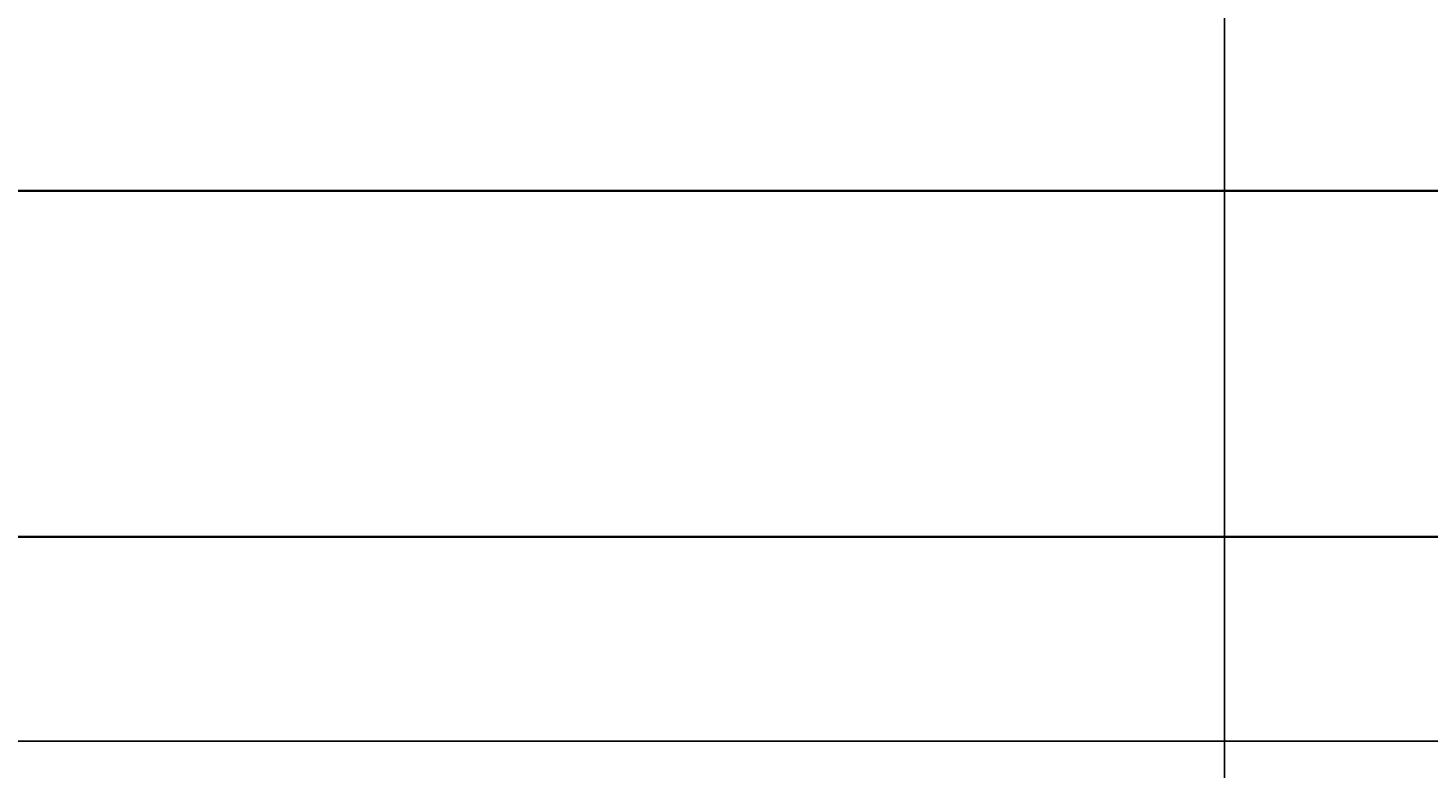
# Model space of a CAD drawing. Units: inches. Extents: x -61 to 1599, y -1316 to 257.
# Tile 49 of 204: x 149 to 185, y -447 to -428. Entities that reach past the tile are written whole.
import ezdxf

# ---------------------------------------------------------------- set-up
doc = ezdxf.new("R2010")
doc.units = ezdxf.units.IN
doc.header["$MEASUREMENT"] = 0
doc.layers.add('A-ANNO-DIMS', color=2, linetype='Continuous', lineweight=18)
doc.layers.add('WALLS', color=4, linetype='Continuous', lineweight=35)
doc.styles.get("Standard").update_dxf_attribs({"font": 'arial.ttf'})
doc.dimstyles.get("Standard").update_dxf_attribs({"dimtxt": 0.18, "dimasz": 0.18, "dimexe": 0.18, "dimexo": 0.0625, "dimgap": 0.09, "dimtad": 0, "dimtih": 1, "dimtoh": 1, "dimdec": 0, "dimzin": 0, "dimdsep": 46, "dimlunit": 3, "dimtxsty": 'Standard', "dimcen": 0.09, "dimadec": 0, "dimazin": 0, "dimtfac": 1, "dimtdec": 0, "dimtofl": 0, "dimtmove": 0, "dimatfit": 3, "dimfxl": 1, "dimtolj": 1, "dimtzin": 0, "dimarcsym": 0})

# ---------------------------------------------------------------- blocks, each defined once
blk = doc.blocks.new('*D687')
at = {"layer": 'A-ANNO-DIMS', "color": 0, "lineweight": -2, "transparency": 16777216}
for p, q in [((289.418, 181.677), (-61.077, 181.677)), ((-60.897, 181.497), (-60.897, -528.952)), ((-60.897, -1239.765), (-60.897, -529.316)), ((319.64, -1239.945), (-61.077, -1239.945))]:
    blk.add_line(p, q, dxfattribs=at)
at = {"layer": 'A-ANNO-DIMS', "color": 0, "transparency": 16777216}
for points in [[(-60.927, 181.497), (-60.867, 181.497), (-60.897, 181.677)], [(-60.927, -1239.765), (-60.867, -1239.765), (-60.897, -1239.945)]]:
    blk.add_solid(points, dxfattribs=at)
at = {"layer": 'DEFPOINTS', "color": 0, "transparency": 16777216}
for p in [(289.481, 181.677), (-60.897, -1239.945), (319.703, -1239.945)]:
    blk.add_point(p, dxfattribs=at)
at = {"layer": 'A-ANNO-DIMS', "color": 0, "transparency": 16777216, "insert": (-60.897, -529.134), "char_height": 0.18, "attachment_point": 5}
blk.add_mtext('\\A1;1421.6', dxfattribs=at)
blk = doc.blocks.new('*D699')
at = {"layer": 'A-ANNO-DIMS', "color": 0, "lineweight": -2, "transparency": 16777216}
for p, q in [((835.64, -167.169), (-61.077, -167.169)), ((-60.897, -167.349), (-60.897, -306.726)), ((-60.897, -446.466), (-60.897, -307.09)), ((841.64, -446.646), (-61.077, -446.646))]:
    blk.add_line(p, q, dxfattribs=at)
at = {"layer": 'A-ANNO-DIMS', "color": 0, "transparency": 16777216}
for points in [[(-60.927, -167.349), (-60.867, -167.349), (-60.897, -167.169)], [(-60.927, -446.466), (-60.867, -446.466), (-60.897, -446.646)]]:
    blk.add_solid(points, dxfattribs=at)
at = {"layer": 'DEFPOINTS', "color": 0, "transparency": 16777216}
for p in [(835.703, -167.169), (-60.897, -446.646), (841.703, -446.646)]:
    blk.add_point(p, dxfattribs=at)
at = {"layer": 'A-ANNO-DIMS', "color": 0, "transparency": 16777216, "insert": (-60.897, -306.908), "char_height": 0.18, "attachment_point": 5}
blk.add_mtext('\\A1;279.5', dxfattribs=at)
blk = doc.blocks.new('*D700')
at = {"layer": 'A-ANNO-DIMS', "color": 0, "lineweight": -2, "transparency": 16777216}
for p, q in [((14.703, -616.882), (14.703, 257.457)), ((14.883, 257.277), (96.772, 257.277)), ((179.572, 257.277), (97.683, 257.277)), ((179.752, -616.882), (179.752, 257.457))]:
    blk.add_line(p, q, dxfattribs=at)
at = {"layer": 'A-ANNO-DIMS', "color": 0, "transparency": 16777216}
for points in [[(14.883, 257.307), (14.883, 257.247), (14.703, 257.277)], [(179.572, 257.307), (179.572, 257.247), (179.752, 257.277)]]:
    blk.add_solid(points, dxfattribs=at)
at = {"layer": 'DEFPOINTS', "color": 0, "transparency": 16777216}
for p in [(179.752, 257.277), (14.703, -616.945), (179.752, -616.945)]:
    blk.add_point(p, dxfattribs=at)
at = {"layer": 'A-ANNO-DIMS', "color": 0, "transparency": 16777216, "insert": (97.227, 257.277), "char_height": 0.18, "attachment_point": 5}
blk.add_mtext('\\A1;165.05', dxfattribs=at)

msp = doc.modelspace()

# ---------------------------------------------------------------- linework, layer by layer
at = {"layer": 'WALLS'}
for p, q in [((87.7028, -432.3229), (237.7028, -432.3229)), ((14.7028, -441.3229), (237.7028, -441.3229))]:
    msp.add_line(p, q, dxfattribs=at)

# ---------------------------------------------------------------- dimensions: what is measured, and where the dimension line sits
at = {"layer": 'A-ANNO-DIMS'}
dim = msp.add_linear_dim(base=(179.7521, 257.2771), p1=(14.7028, -616.9446), p2=(179.7521, -616.9446), dimstyle='Standard', override={"dimdec": 2, "dimlfac": 1, "dimrnd": 0, "dimzin": 0, "dimdsep": 46, "dimlunit": 2}, dxfattribs=at)
dim.commit()
dim.dimension.update_dxf_attribs({"geometry": '*D700', "text_midpoint": (97.2274, 257.2771)})
for base, p1, p2, picture, middle in [((-60.8972, -1239.9446), (289.4807, 181.6771), (319.7028, -1239.9446), '*D687', (-60.8972, -529.1337)), ((-60.8972, -446.6462), (835.7028, -167.169), (841.7028, -446.6462), '*D699', (-60.8972, -306.9076))]:
    dim = msp.add_linear_dim(base=base, p1=p1, p2=p2, angle=90, dimstyle='Standard', override={"dimdec": 1, "dimlfac": 1, "dimrnd": 0, "dimzin": 0, "dimdsep": 46, "dimlunit": 2}, dxfattribs=at)
    dim.commit()
    dim.dimension.update_dxf_attribs({"geometry": picture, "text_midpoint": middle})

doc.saveas('drawing.dxf')
